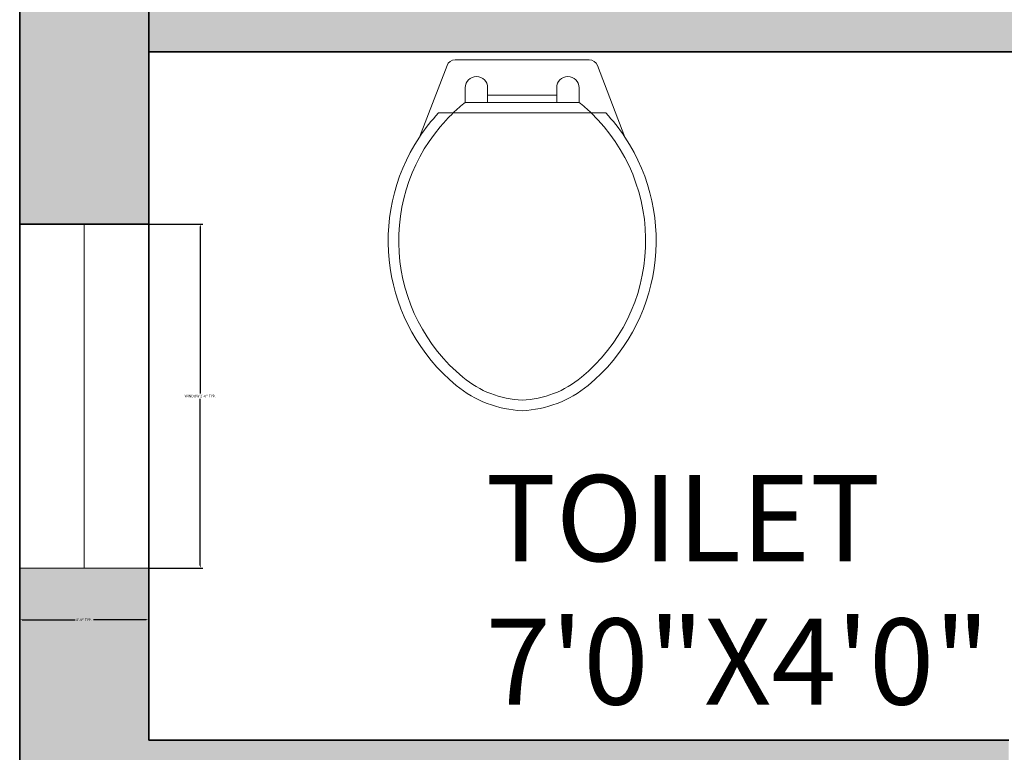
# Model space of a CAD drawing. Units: inches. Extents: x -9 to 505, y -680 to 48.
# Tile 12 of 17: x 27 to 96, y -165 to -114. Entities that reach past the tile are written whole.
import ezdxf

# ---------------------------------------------------------------- set-up
doc = ezdxf.new("R2010")
doc.units = ezdxf.units.IN
doc.header["$MEASUREMENT"] = 0
for name, color, linetype, lineweight in [('A-ANNO-DIMS', 2, 'Continuous', 18), ('A-AREA-IDEN', 7, 'Continuous', 18), ('A-GLAZ', 4, 'Continuous', 18), ('A-WALL', 7, 'Continuous', 35), ('A-WALL-PATT', 251, 'Continuous', 13), ('S-CONC', 7, 'Continuous', 35), ('S-CONC-PATT', 18, 'Continuous', 13), ('WC-Detail_dwgmodels.com', 251, 'Continuous', 13), ('WC-Outline_dwgmodels.com', 250, 'Continuous', 18)]:
    doc.layers.add(name, color=color, linetype=linetype, lineweight=lineweight)
doc.styles.get("Standard").update_dxf_attribs({"font": 'arial.ttf'})
doc.dimstyles.get("Standard").update_dxf_attribs({"dimtxt": 0.18, "dimasz": 0.18, "dimexe": 0.18, "dimexo": 0.0625, "dimgap": 0.09, "dimtad": 0, "dimtih": 1, "dimtoh": 1, "dimdec": 0, "dimzin": 0, "dimdsep": 46, "dimlunit": 3, "dimtxsty": 'Standard', "dimcen": 0.09, "dimadec": 0, "dimazin": 0, "dimtfac": 1, "dimtdec": 0, "dimtofl": 0, "dimtmove": 0, "dimatfit": 3, "dimfxl": 1, "dimtolj": 1, "dimtzin": 0, "dimarcsym": 0})

# ---------------------------------------------------------------- blocks, each defined once
blk = doc.blocks.new('*D3')
at = {"layer": 'A-ANNO-DIMS', "color": 0, "lineweight": -2, "transparency": 16777216}
for p, q in [((27.201, 11.499), (5.161, 11.499)), ((5.341, 11.319), (5.341, -330.86)), ((5.341, -679.321), (5.341, -337.142)), ((27.201, -679.501), (5.161, -679.501))]:
    blk.add_line(p, q, dxfattribs=at)
at = {"layer": 'A-ANNO-DIMS', "color": 0, "transparency": 16777216}
for points in [[(5.311, 11.319), (5.371, 11.319), (5.341, 11.499)], [(5.311, -679.321), (5.371, -679.321), (5.341, -679.501)]]:
    blk.add_solid(points, dxfattribs=at)
at = {"layer": 'Defpoints', "color": 0, "transparency": 16777216}
for p in [(27.264, 11.499), (5.341, -679.501), (27.264, -679.501)]:
    blk.add_point(p, dxfattribs=at)
at = {"layer": 'A-ANNO-DIMS', "color": 0, "transparency": 16777216, "insert": (5.341, -334.001), "char_height": 6, "attachment_point": 5}
blk.add_mtext('\\A1;57\'-7"', dxfattribs=at)
blk = doc.blocks.new('WIN-24')
for p, q in [((0, 24), (0, 0)), ((9, 24), (0, 24)), ((4.5, 24), (4.5, 2.228)), ((9, 0), (9, 24)), ((4.5, 2.228), (4.5, 0)), ((0, 0), (9, 0))]:
    blk.add_line(p, q)
blk = doc.blocks.new('*D18')
at = {"layer": 'A-ANNO-DIMS', "color": 0, "lineweight": -2, "transparency": 16777216}
for p, q in [((36.326, -128.001), (40.044, -128.001)), ((39.864, -128.181), (39.864, -139.818)), ((39.864, -151.821), (39.864, -140.184)), ((36.326, -152.001), (40.044, -152.001))]:
    blk.add_line(p, q, dxfattribs=at)
at = {"layer": 'A-ANNO-DIMS', "color": 0, "transparency": 16777216}
for points in [[(39.834, -128.181), (39.894, -128.181), (39.864, -128.001)], [(39.834, -151.821), (39.894, -151.821), (39.864, -152.001)]]:
    blk.add_solid(points, dxfattribs=at)
at = {"layer": 'Defpoints', "color": 0, "transparency": 16777216}
for p in [(36.264, -128.001), (39.864, -128.001), (36.264, -152.001)]:
    blk.add_point(p, dxfattribs=at)
at = {"layer": 'A-ANNO-DIMS', "color": 0, "transparency": 16777216, "insert": (39.864, -140.001), "char_height": 0.18, "attachment_point": 5}
blk.add_mtext('\\A1;WINDOW 2\'-0" TYP.', dxfattribs=at)
blk = doc.blocks.new('*D19')
at = {"layer": 'A-ANNO-DIMS', "color": 0, "lineweight": -2, "transparency": 16777216}
for p, q in [((27.264, -152.063), (27.264, -155.781)), ((36.264, -152.063), (36.264, -155.781)), ((27.444, -155.601), (31.125, -155.601)), ((36.084, -155.601), (32.402, -155.601))]:
    blk.add_line(p, q, dxfattribs=at)
at = {"layer": 'A-ANNO-DIMS', "color": 0, "transparency": 16777216}
for points in [[(27.444, -155.571), (27.444, -155.631), (27.264, -155.601)], [(36.084, -155.571), (36.084, -155.631), (36.264, -155.601)]]:
    blk.add_solid(points, dxfattribs=at)
at = {"layer": 'Defpoints', "color": 0, "transparency": 16777216}
for p in [(27.264, -152.001), (36.264, -152.001), (36.264, -155.601)]:
    blk.add_point(p, dxfattribs=at)
at = {"layer": 'A-ANNO-DIMS', "color": 0, "transparency": 16777216, "insert": (31.764, -155.601), "char_height": 0.18, "attachment_point": 5}
blk.add_mtext('\\A1;0\'-9" TYP.', dxfattribs=at)

msp = doc.modelspace()

# ---------------------------------------------------------------- hatches: boundary and pattern name
at = {"layer": 'A-WALL-PATT'}
h = msp.add_hatch(color=256, dxfattribs=at)
h.dxf.hatch_style = 1
h.paths.add_polyline_path([(101.641, 11.499), (48.264, 11.499), (48.264, 2.499), (72.264, 2.499), (72.264, -21.248), (81.264, -21.248), (81.264, 2.499), (101.641, 2.499)])
h.paths.add_polyline_path([(36.264, 2.499), (27.264, 2.499), (27.264, -6.918), (36.264, -6.918)])
h.paths.add_polyline_path([(81.264, -57.248), (72.264, -57.248), (72.264, -75.501), (81.264, -75.501)])
h.paths.add_polyline_path([(162.764, 11.499), (137.641, 11.499), (137.641, 2.499), (162.764, 2.499)])
h.paths.add_polyline_path([(179.264, 2.499), (174.764, 2.499), (174.764, -75.501), (179.264, -75.501), (179.264, -54.501), (229.514, -54.501), (229.514, -45.501), (179.264, -45.501)])
h.paths.add_polyline_path([(382.256, -45.501), (332.264, -45.501), (332.264, 2.499), (327.764, 2.499), (327.764, -45.501), (277.514, -45.501), (277.514, -54.501), (327.764, -54.501), (327.764, -111.501), (332.264, -111.501), (332.264, -54.501), (382.256, -54.501)])
h.paths.add_polyline_path([(332.264, -128.001), (327.764, -128.001), (327.764, -207.001), (332.264, -207.001)])
h.paths.add_polyline_path([(124.764, -111.501), (36.264, -111.501), (36.264, -116.001), (120.264, -116.001), (120.264, -168.501), (179.264, -168.501), (179.264, -164.001), (124.764, -164.001)])
h.paths.add_polyline_path([(96.264, -164.001), (36.264, -164.001), (36.264, -152.001), (27.264, -152.001), (27.264, -208.879), (36.264, -208.879), (36.264, -168.501), (96.264, -168.501)])
h.paths.add_polyline_path([(36.264, -244.879), (27.264, -244.879), (27.264, -287.001), (36.264, -287.001)])
h.paths.add_polyline_path([(179.264, -204.501), (174.764, -204.501), (174.764, -287.001), (179.264, -287.001)])
h.paths.add_polyline_path([(257.264, -296.001), (248.264, -296.001), (248.264, -446.001), (269.264, -446.001), (269.264, -437.001), (257.264, -437.001)])
h.paths.add_polyline_path([(90.264, -296.001), (81.264, -296.001), (81.264, -348.67), (90.264, -348.67)])
h.paths.add_polyline_path([(90.264, -384.67), (81.264, -384.67), (81.264, -416.001), (90.264, -416.001)])
h.paths.add_polyline_path([(170.264, -452.001), (36.264, -452.001), (36.264, -456.501), (165.764, -456.501), (165.764, -504.501), (165.133, -504.501), (165.133, -509.001), (170.264, -509.001)])
h.paths.add_polyline_path([(141.764, -504.501), (36.264, -504.501), (36.264, -492.501), (27.264, -492.501), (27.264, -565.959), (36.264, -565.959), (36.264, -509.001), (141.764, -509.001)])
h.paths.add_polyline_path([(36.264, -601.959), (27.264, -601.959), (27.264, -658.501), (36.264, -658.501)])
h.paths.add_polyline_path([(170.264, -670.501), (170.264, -634.501), (222.764, -634.501), (222.764, -625.501), (165.764, -625.501), (165.764, -670.501), (36.264, -670.501), (36.264, -679.501), (170.264, -679.501)])
h.paths.add_polyline_path([(332.264, -616.501), (433.894, -616.501), (433.894, -612.001), (332.264, -612.001), (332.264, -610.563), (327.764, -610.563), (327.764, -625.501), (270.764, -625.501), (270.764, -634.501), (327.764, -634.501), (327.764, -658.501), (332.264, -658.501)])
h.paths.add_polyline_path([(459.764, -670.501), (336.764, -670.501), (336.764, -679.501), (459.764, -679.501)])
h.paths.add_polyline_path([(468.764, -545.737), (459.764, -545.737), (459.764, -612.001), (457.894, -612.001), (457.894, -616.501), (459.764, -616.501), (459.764, -658.501), (468.764, -658.501)])
h.paths.add_polyline_path([(332.264, -446.001), (327.764, -446.001), (327.764, -574.563), (332.264, -574.563)])
h.paths.add_polyline_path([(327.764, -437.001), (305.264, -437.001), (305.264, -446.001), (327.764, -446.001)])
h.paths.add_polyline_path([(459.764, -437.001), (348.764, -437.001), (348.764, -446.001), (459.764, -446.001)])
h.paths.add_polyline_path([(468.764, -458.001), (459.764, -458.001), (459.764, -509.737), (468.764, -509.737)])
h.paths.add_polyline_path([(468.764, -365.001), (459.764, -365.001), (459.764, -437.001), (468.764, -437.001)])
h.paths.add_polyline_path([(468.764, -299.601), (459.764, -299.601), (459.764, -344.001), (468.764, -344.001)])
h.paths.add_polyline_path([(468.764, -184.739), (459.764, -184.739), (459.764, -231.001), (401.264, -231.001), (401.264, -235.501), (459.764, -235.501), (459.764, -275.601), (468.764, -275.601)])
h.paths.add_polyline_path([(390.764, -356.001), (342.764, -356.001), (342.764, -365.001), (390.764, -365.001)])
h.paths.add_polyline_path([(459.764, -356.001), (405.764, -356.001), (405.764, -365.001), (459.764, -365.001)])
h.paths.add_polyline_path([(405.764, -296.001), (396.764, -296.001), (396.764, -356.001), (405.764, -356.001)])
h.paths.add_polyline_path([(336.764, -296.001), (327.764, -296.001), (327.764, -356.001), (336.764, -356.001)])
h.paths.add_polyline_path([(468.764, -9.501), (459.764, -9.501), (459.764, -45.501), (418.256, -45.501), (418.256, -54.501), (468.764, -54.501)])
h.paths.add_polyline_path([(468.764, -54.501), (459.764, -54.501), (459.764, -111.501), (468.764, -111.501)])
h.paths.add_polyline_path([(468.764, -128.001), (459.764, -128.001), (459.764, -148.739), (468.764, -148.739)])
at = {"layer": 'S-CONC-PATT'}
h = msp.add_hatch(color=256, dxfattribs=at)
h.dxf.hatch_style = 1
h.paths.add_polyline_path([(36.264, -111.501), (27.264, -111.501), (27.264, -128.001), (36.264, -128.001)])

# ---------------------------------------------------------------- linework, layer by layer
at = {"layer": 'A-WALL'}
for p, q in [((27.264, 11.499), (27.264, -679.501)), ((36.264, 2.499), (36.264, -164.001)), ((36.264, -116.001), (120.264, -116.001)), ((36.264, -164.001), (96.264, -164.001))]:
    msp.add_line(p, q, dxfattribs=at)
at = {"layer": 'S-CONC'}
msp.add_line((36.264, -128.001), (27.264, -128.001), dxfattribs=at)
at = {"layer": 'WC-Detail_dwgmodels.com'}
for p, q in [((56.48, -120.256), (57.506, -120.256)), ((67.132, -120.256), (68.158, -120.256))]:
    msp.add_line(p, q, dxfattribs=at)
for points in [[(58.35, -119.517), (58.35, -118.491, -1), (59.91, -118.491), (59.91, -119.025)], [(66.288, -119.517), (66.288, -118.491, 1), (64.728, -118.491), (64.728, -119.025)], [(58.35, -119.517, 0.022712), (57.506, -120.256, 0.162618)], [(62.319, -119.517), (58.35, -119.517, 0.022712)], [(62.319, -119.517), (66.288, -119.517, -0.476108)], [(66.288, -119.517, -0.022712), (67.132, -120.256, -0.162618)], [(56.48, -120.256, 0.040937), (55.155, -121.935, 0.163732)], [(68.158, -120.256, -0.040937), (69.483, -121.935, -0.163732)]]:
    msp.add_lwpolyline(points, format="xyb", dxfattribs=at)
for points in [[(64.728, -119.025), (59.91, -119.025)], [(59.91, -119.025), (59.91, -119.517)], [(64.728, -119.025), (64.728, -119.517)]]:
    msp.add_lwpolyline(points, dxfattribs=at)
at = {"layer": 'WC-Outline_dwgmodels.com'}
for p in [(57.506, -120.256), (67.132, -120.256)]:
    msp.add_line(p, (62.319, -120.256), dxfattribs=at)
for points in [[(62.319, -116.552), (57.647, -116.552, 0.31031), (57.075, -116.945), (55.155, -121.935, 0.209071)], [(62.319, -116.552), (66.991, -116.552, -0.31031), (67.563, -116.945), (69.483, -121.935, -0.209071)], [(57.015, -120.754, 0.431639), (58.186, -138.69, 0.162618), (62.319, -140.285, 0.470877)], [(57.506, -120.256, 0.014165), (57.015, -120.754, 0.162618)], [(67.132, -120.256, -0.448546), (66.452, -138.69, -0.162618), (62.319, -140.285, -0.470877)], [(55.155, -121.935, 0.383919), (57.72, -139.254, 0.163732), (62.319, -141.017, 0.359733)], [(69.483, -121.935, -0.383919), (66.918, -139.254, -0.163732), (62.319, -141.017, -0.359733)]]:
    msp.add_lwpolyline(points, format="xyb", dxfattribs=at)

# ---------------------------------------------------------------- block references
at = {"layer": 'A-GLAZ'}
msp.add_blockref('WIN-24', (27.264, -152.001), dxfattribs=at)

# ---------------------------------------------------------------- texts
at = {"layer": 'A-AREA-IDEN', "insert": (59.768, -145.513), "char_height": 6, "attachment_point": 1}
msp.add_mtext('TOILET\\P7\'0"X4\'0"', dxfattribs=at)

# ---------------------------------------------------------------- dimensions: what is measured, and where the dimension line sits
at = {"layer": 'A-ANNO-DIMS'}
dim = msp.add_linear_dim(base=(5.341, -679.501), p1=(27.264, 11.499), p2=(27.264, -679.501), angle=90, dimstyle='Standard', override={"dimtxt": 6, "dimclrd": 0, "dimclre": 0, "dimclrt": 0}, dxfattribs=at)
dim.commit()
dim.dimension.update_dxf_attribs({"geometry": '*D3', "text_midpoint": (5.341, -334.001)})
dim = msp.add_linear_dim(base=(39.864, -128.001), p1=(36.264, -152.001), p2=(36.264, -128.001), angle=90, text='WINDOW <> TYP.', dimstyle='Standard', override={"dimdec": 1, "dimlfac": 1, "dimrnd": 0, "dimzin": 1, "dimdsep": 46, "dimlunit": 4, "dimfrac": 2}, dxfattribs=at)
dim.commit()
dim.dimension.update_dxf_attribs({"geometry": '*D18', "text_midpoint": (39.864, -140.001)})
dim = msp.add_linear_dim(base=(36.264, -155.601), p1=(27.264, -152.001), p2=(36.264, -152.001), text='<> TYP.', dimstyle='Standard', override={"dimdec": 1, "dimlfac": 1, "dimrnd": 0, "dimzin": 1, "dimdsep": 46, "dimlunit": 4, "dimfrac": 2}, dxfattribs=at)
dim.commit()
dim.dimension.update_dxf_attribs({"geometry": '*D19', "text_midpoint": (31.764, -155.601)})

doc.saveas('drawing.dxf')
